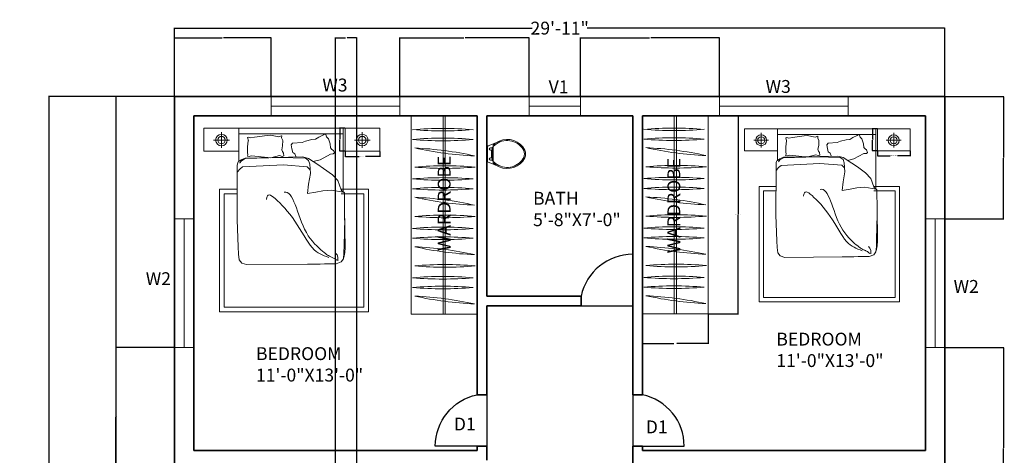
# Model space of a CAD drawing. Units: inches. Extents: x -53 to 406, y -526 to 46.
# Tile 2 of 2: x -53 to 406, y -157 to 46. Entities that reach past the tile are written whole.
import ezdxf

# ---------------------------------------------------------------- set-up
doc = ezdxf.new("R2010")
doc.units = ezdxf.units.IN
doc.header["$MEASUREMENT"] = 0
for name, color, linetype, lineweight in [('A-ANNO-DIMS', 2, 'Continuous', 18), ('A-ANNO-TEXT', 7, 'Continuous', 18), ('A-AREA-IDEN', 7, 'Continuous', 25), ('A-DOOR', 40, 'Continuous', 25), ('A-FLOR-CASE', 9, 'Continuous', 18), ('A-FURN', 8, 'Continuous', 13), ('A-GLAZ', 175, 'Continuous', 18), ('A-WALL', 7, 'Continuous', 35), ('WC-Detail_dwgmodels.com', 251, 'Continuous', 13), ('WC-Outline_dwgmodels.com', 250, 'Continuous', 18)]:
    doc.layers.add(name, color=color, linetype=linetype, lineweight=lineweight)
doc.styles.get("Standard").update_dxf_attribs({"font": 'arial.ttf'})
doc.dimstyles.get("Standard").update_dxf_attribs({"dimtxt": 0.18, "dimasz": 0.18, "dimexe": 0.18, "dimexo": 0.0625, "dimgap": 0.09, "dimtad": 0, "dimtih": 1, "dimtoh": 1, "dimdec": 0, "dimzin": 0, "dimdsep": 46, "dimlunit": 3, "dimtxsty": 'Standard', "dimcen": 0.09, "dimadec": 0, "dimazin": 0, "dimtfac": 1, "dimtdec": 0, "dimtofl": 0, "dimtmove": 0, "dimatfit": 3, "dimfxl": 1, "dimtolj": 1, "dimtzin": 0, "dimarcsym": 0})

# ---------------------------------------------------------------- blocks, each defined once
blk = doc.blocks.new('*D1')
at = {"layer": 'A-ANNO-DIMS', "color": 0, "lineweight": -2, "transparency": 16777216}
for p, q in [((19.43, 9.97), (19.43, 42.02)), ((19.61, 41.84), (186.15, 41.84)), ((378.25, 41.84), (211.71, 41.84)), ((378.43, 9.97), (378.43, 42.02))]:
    blk.add_line(p, q, dxfattribs=at)
at = {"layer": 'A-ANNO-DIMS', "color": 0, "transparency": 16777216}
for points in [[(19.61, 41.87), (19.61, 41.81), (19.43, 41.84)], [(378.25, 41.87), (378.25, 41.81), (378.43, 41.84)]]:
    blk.add_solid(points, dxfattribs=at)
at = {"layer": 'Defpoints', "color": 0, "transparency": 16777216}
for p in [(378.43, 41.84), (19.43, 9.91), (378.43, 9.91)]:
    blk.add_point(p, dxfattribs=at)
at = {"layer": 'A-ANNO-DIMS', "color": 0, "transparency": 16777216, "insert": (198.93, 41.84), "char_height": 6, "attachment_point": 5}
blk.add_mtext('\\A1;29\'-11"', dxfattribs=at)
blk = doc.blocks.new('*D2')
at = {"layer": 'A-ANNO-DIMS', "color": 0, "lineweight": -2, "transparency": 16777216}
for p, q in [((19.37, 9.91), (-39.35, 9.91)), ((-39.17, 9.73), (-39.17, -226.19)), ((-39.17, -468.41), (-39.17, -232.5)), ((19.37, -468.59), (-39.35, -468.59))]:
    blk.add_line(p, q, dxfattribs=at)
at = {"layer": 'A-ANNO-DIMS', "color": 0, "transparency": 16777216}
for points in [[(-39.2, 9.73), (-39.14, 9.73), (-39.17, 9.91)], [(-39.2, -468.41), (-39.14, -468.41), (-39.17, -468.59)]]:
    blk.add_solid(points, dxfattribs=at)
at = {"layer": 'Defpoints', "color": 0, "transparency": 16777216}
for p in [(19.43, 9.91), (-39.17, -468.59), (19.43, -468.59)]:
    blk.add_point(p, dxfattribs=at)
at = {"layer": 'A-ANNO-DIMS', "color": 0, "transparency": 16777216, "insert": (-39.17, -229.34), "char_height": 6, "attachment_point": 5}
blk.add_mtext('\\A1;39\'-11"', dxfattribs=at)
blk = doc.blocks.new('WIN-60IN-9IN-WALL')
for p, q in [((60, 9), (0, 9)), ((0, 9), (0, 0)), ((60, 0), (60, 9)), ((0, 4.5), (60, 4.5)), ((0, 0), (60, 0))]:
    blk.add_line(p, q)
blk = doc.blocks.new('VENT-24IN-9IN-WALL')
for p, q in [((24, 9), (0, 9)), ((0, 9), (0, 0)), ((24, 0), (24, 9)), ((0, 4.5), (24, 4.5)), ((0, 0), (24, 0))]:
    blk.add_line(p, q)
blk = doc.blocks.new('DOOR-24IN-SINGLE')
for p, q in [((24, 0), (24, 24)), ((0, 0), (24, 0))]:
    blk.add_line(p, q)
blk.add_arc((24, -0.52), 24.52, 90, 168.1877)
blk = doc.blocks.new('WARDROBE-HANGING')
for p, q in [((0, 0), (0, 92.26)), ((30.75, 92.26), (0, 92.26)), ((14.86, 0), (14.86, 92.26)), ((15.89, 0), (15.89, 92.26)), ((30.75, 0), (30.75, 92.26)), ((30.75, 0), (0, 0))]:
    blk.add_line(p, q)
for centre, start, end in [((14.76, -75.2), 85.0028, 94.9972), ((14.76, 247.2), 265.0028, 274.9972), ((14.76, -79.75), 85.0028, 94.9972), ((14.76, 242.64), 265.0028, 274.9972), ((36.65, 235.44), 257.508, 267.5023), ((-5.4, -84.2), 77.508, 87.5023), ((15.75, -92.64), 85.0028, 94.9972), ((15.75, 229.75), 265.0028, 274.9972), ((14.76, -98.18), 85.0028, 94.9972), ((14.76, 224.21), 265.0028, 274.9972), ((14.76, -102.74), 85.0028, 94.9972), ((14.76, 219.65), 265.0028, 274.9972), ((36.65, 212.45), 257.508, 267.5023), ((-5.4, -107.18), 77.508, 87.5023), ((15.75, -115.63), 85.0028, 94.9972), ((15.75, 206.76), 265.0028, 274.9972), ((14.76, -121.25), 85.0028, 94.9972), ((14.76, 201.14), 265.0028, 274.9972), ((14.76, -125.81), 85.0028, 94.9972), ((14.76, 196.58), 265.0028, 274.9972), ((-5.4, -130.25), 77.508, 87.5023), ((36.65, 189.38), 257.508, 267.5023), ((15.75, -138.7), 85.0028, 94.9972), ((15.75, 183.69), 265.0028, 274.9972), ((14.76, -144.24), 85.0028, 94.9972), ((14.76, 178.15), 265.0028, 274.9972), ((14.76, -148.79), 85.0028, 94.9972), ((14.76, 173.6), 265.0028, 274.9972), ((-5.4, -153.24), 77.508, 87.5023), ((36.65, 166.4), 257.508, 267.5023)]:
    blk.add_arc(centre, 161.81, start, end)
blk = doc.blocks.new('NIGHTSTAND-15IN')
for p, q in [((4.25, 4.91), (11.18, 4.91)), ((7.71, 8.38), (7.71, 1.45))]:
    blk.add_line(p, q)
blk.add_lwpolyline([(0, 0), (15.27, 0), (15.27, 10.18), (0, 10.18)], close=True)
for radius in [2.55, 1.63]:
    blk.add_circle((7.71, 4.91), radius)
blk = doc.blocks.new('NIGHTSTAND-16IN')
for p, q in [((4.52, 5.22), (11.88, 5.22)), ((8.2, 8.9), (8.2, 1.54))]:
    blk.add_line(p, q)
blk.add_lwpolyline([(0, 0), (16.23, 0), (16.23, 10.82), (0, 10.82)], close=True)
for radius in [2.71, 1.73]:
    blk.add_circle((8.2, 5.22), radius)
blk = doc.blocks.new('*D15')
at = {"layer": 'A-ANNO-DIMS', "color": 0, "lineweight": -2, "transparency": 16777216}
for p, q in [((268.25, 0.91), (282.2, 0.91)), ((282.02, 0.73), (282.02, -45.04)), ((282.02, -91.17), (282.02, -45.4)), ((268.25, -91.35), (282.2, -91.35))]:
    blk.add_line(p, q, dxfattribs=at)
at = {"layer": 'A-ANNO-DIMS', "color": 0, "transparency": 16777216}
for points in [[(281.99, 0.73), (282.05, 0.73), (282.02, 0.91)], [(281.99, -91.17), (282.05, -91.17), (282.02, -91.35)]]:
    blk.add_solid(points, dxfattribs=at)
at = {"layer": 'Defpoints', "color": 0, "transparency": 16777216}
for p in [(268.18, 0.91), (282.02, 0.91), (268.18, -91.35)]:
    blk.add_point(p, dxfattribs=at)
at = {"layer": 'A-ANNO-DIMS', "color": 0, "transparency": 16777216, "insert": (282.02, -45.22), "char_height": 0.18, "attachment_point": 5}
blk.add_mtext('\\A1;WARDROBE 7\'-8 1/2" TYP.', dxfattribs=at)
blk = doc.blocks.new('*D16')
at = {"layer": 'A-ANNO-DIMS', "color": 0, "lineweight": -2, "transparency": 16777216}
for p, q in [((237.43, -91.41), (237.43, -105.37)), ((268.18, -91.41), (268.18, -105.37)), ((237.61, -105.19), (252.17, -105.19)), ((268, -105.19), (253.45, -105.19))]:
    blk.add_line(p, q, dxfattribs=at)
at = {"layer": 'A-ANNO-DIMS', "color": 0, "transparency": 16777216}
for points in [[(237.61, -105.16), (237.61, -105.22), (237.43, -105.19)], [(268, -105.16), (268, -105.22), (268.18, -105.19)]]:
    blk.add_solid(points, dxfattribs=at)
at = {"layer": 'Defpoints', "color": 0, "transparency": 16777216}
for p in [(237.43, -91.35), (268.18, -91.35), (268.18, -105.19)]:
    blk.add_point(p, dxfattribs=at)
at = {"layer": 'A-ANNO-DIMS', "color": 0, "transparency": 16777216, "insert": (252.81, -105.19), "char_height": 0.18, "attachment_point": 5}
blk.add_mtext('\\A1;2\'-7" TYP.', dxfattribs=at)
blk = doc.blocks.new('*D17')
at = {"layer": 'A-ANNO-DIMS', "color": 0, "lineweight": -2, "transparency": 16777216}
for p, q in [((347.01, -15.4), (347.01, -17.81)), ((347.19, -17.63), (352.94, -17.63)), ((362.09, -17.63), (356.34, -17.63)), ((362.27, -15.4), (362.27, -17.81))]:
    blk.add_line(p, q, dxfattribs=at)
at = {"layer": 'A-ANNO-DIMS', "color": 0, "transparency": 16777216}
for points in [[(347.19, -17.6), (347.19, -17.66), (347.01, -17.63)], [(362.09, -17.6), (362.09, -17.66), (362.27, -17.63)]]:
    blk.add_solid(points, dxfattribs=at)
at = {"layer": 'Defpoints', "color": 0, "transparency": 16777216}
for p in [(347.01, -15.34), (347.01, -17.63), (362.27, -15.34)]:
    blk.add_point(p, dxfattribs=at)
at = {"layer": 'A-ANNO-DIMS', "color": 0, "transparency": 16777216, "insert": (354.64, -17.63), "char_height": 0.18, "attachment_point": 5}
blk.add_mtext('\\A1;NIGHTSTAND 1\'-3 1/2" TYP.', dxfattribs=at)
blk = doc.blocks.new('*D18')
at = {"layer": 'A-ANNO-DIMS', "color": 0, "lineweight": -2, "transparency": 16777216}
for p, q in [((346.95, -5.16), (344.54, -5.16)), ((344.72, -5.34), (344.72, -10.07)), ((344.72, -15.16), (344.72, -10.43)), ((346.95, -15.34), (344.54, -15.34))]:
    blk.add_line(p, q, dxfattribs=at)
at = {"layer": 'A-ANNO-DIMS', "color": 0, "transparency": 16777216}
for points in [[(344.69, -5.34), (344.75, -5.34), (344.72, -5.16)], [(344.69, -15.16), (344.75, -15.16), (344.72, -15.34)]]:
    blk.add_solid(points, dxfattribs=at)
at = {"layer": 'Defpoints', "color": 0, "transparency": 16777216}
for p in [(344.72, -5.16), (347.01, -5.16), (347.01, -15.34)]:
    blk.add_point(p, dxfattribs=at)
at = {"layer": 'A-ANNO-DIMS', "color": 0, "transparency": 16777216, "insert": (344.72, -10.25), "char_height": 0.18, "attachment_point": 5}
blk.add_mtext('\\A1;0\'-10" TYP.', dxfattribs=at)
blk = doc.blocks.new('*D19')
at = {"layer": 'A-ANNO-DIMS', "color": 0, "lineweight": -2, "transparency": 16777216}
for p, q in [((98.87, -15.63), (98.87, -18.18)), ((99.05, -18), (105.5, -18)), ((114.92, -18), (108.47, -18)), ((115.1, -15.63), (115.1, -18.18))]:
    blk.add_line(p, q, dxfattribs=at)
at = {"layer": 'A-ANNO-DIMS', "color": 0, "transparency": 16777216}
for points in [[(99.05, -17.97), (99.05, -18.03), (98.87, -18)], [(114.92, -17.97), (114.92, -18.03), (115.1, -18)]]:
    blk.add_solid(points, dxfattribs=at)
at = {"layer": 'Defpoints', "color": 0, "transparency": 16777216}
for p in [(98.87, -15.57), (98.87, -18), (115.1, -15.57)]:
    blk.add_point(p, dxfattribs=at)
at = {"layer": 'A-ANNO-DIMS', "color": 0, "transparency": 16777216, "insert": (106.98, -18), "char_height": 0.18, "attachment_point": 5}
blk.add_mtext('\\A1;NIGHTSTAND 1\'-4" TYP.', dxfattribs=at)
blk = doc.blocks.new('*D20')
at = {"layer": 'A-ANNO-DIMS', "color": 0, "lineweight": -2, "transparency": 16777216}
for p, q in [((98.81, -4.75), (96.26, -4.75)), ((96.44, -4.93), (96.44, -9.98)), ((96.44, -15.39), (96.44, -10.34)), ((98.81, -15.57), (96.26, -15.57))]:
    blk.add_line(p, q, dxfattribs=at)
at = {"layer": 'A-ANNO-DIMS', "color": 0, "transparency": 16777216}
for points in [[(96.41, -4.93), (96.47, -4.93), (96.44, -4.75)], [(96.41, -15.39), (96.47, -15.39), (96.44, -15.57)]]:
    blk.add_solid(points, dxfattribs=at)
at = {"layer": 'Defpoints', "color": 0, "transparency": 16777216}
for p in [(96.44, -4.75), (98.87, -4.75), (98.87, -15.57)]:
    blk.add_point(p, dxfattribs=at)
at = {"layer": 'A-ANNO-DIMS', "color": 0, "transparency": 16777216, "insert": (96.44, -10.16), "char_height": 0.18, "attachment_point": 5}
blk.add_mtext('\\A1;0\'-11" TYP.', dxfattribs=at)
blk = doc.blocks.new('*D22')
at = {"layer": 'A-ANNO-DIMS', "color": 0, "lineweight": -2, "transparency": 16777216}
for p, q in [((19.43, 9.97), (19.43, 37.44)), ((19.61, 37.26), (41.6, 37.26)), ((64.25, 37.26), (42.26, 37.26)), ((64.43, 9.97), (64.43, 37.44))]:
    blk.add_line(p, q, dxfattribs=at)
at = {"layer": 'A-ANNO-DIMS', "color": 0, "transparency": 16777216}
for points in [[(19.61, 37.29), (19.61, 37.23), (19.43, 37.26)], [(64.25, 37.29), (64.25, 37.23), (64.43, 37.26)]]:
    blk.add_solid(points, dxfattribs=at)
at = {"layer": 'Defpoints', "color": 0, "transparency": 16777216}
for p in [(64.43, 37.26), (19.43, 9.91), (64.43, 9.91)]:
    blk.add_point(p, dxfattribs=at)
at = {"layer": 'A-ANNO-DIMS', "color": 0, "transparency": 16777216, "insert": (41.93, 37.26), "char_height": 0.18, "attachment_point": 5}
blk.add_mtext('\\A1;3\'-9"', dxfattribs=at)
blk = doc.blocks.new('*D23')
at = {"layer": 'A-ANNO-DIMS', "color": 0, "lineweight": -2, "transparency": 16777216}
for p, q in [((124.43, 9.97), (124.43, 37.44)), ((124.61, 37.26), (154.23, 37.26)), ((184.5, 37.26), (154.88, 37.26)), ((184.68, 9.97), (184.68, 37.44))]:
    blk.add_line(p, q, dxfattribs=at)
at = {"layer": 'A-ANNO-DIMS', "color": 0, "transparency": 16777216}
for points in [[(124.61, 37.29), (124.61, 37.23), (124.43, 37.26)], [(184.5, 37.29), (184.5, 37.23), (184.68, 37.26)]]:
    blk.add_solid(points, dxfattribs=at)
at = {"layer": 'Defpoints', "color": 0, "transparency": 16777216}
for p in [(184.68, 37.26), (124.43, 9.91), (184.68, 9.91)]:
    blk.add_point(p, dxfattribs=at)
at = {"layer": 'A-ANNO-DIMS', "color": 0, "transparency": 16777216, "insert": (154.56, 37.26), "char_height": 0.18, "attachment_point": 5}
blk.add_mtext('\\A1;5\'-0"', dxfattribs=at)
blk = doc.blocks.new('*D24')
at = {"layer": 'A-ANNO-DIMS', "color": 0, "lineweight": -2, "transparency": 16777216}
for p, q in [((208.68, 9.97), (208.68, 37.44)), ((208.86, 37.26), (240.73, 37.26)), ((273.25, 37.26), (241.38, 37.26)), ((273.43, 9.97), (273.43, 37.44))]:
    blk.add_line(p, q, dxfattribs=at)
at = {"layer": 'A-ANNO-DIMS', "color": 0, "transparency": 16777216}
for points in [[(208.86, 37.29), (208.86, 37.23), (208.68, 37.26)], [(273.25, 37.29), (273.25, 37.23), (273.43, 37.26)]]:
    blk.add_solid(points, dxfattribs=at)
at = {"layer": 'Defpoints', "color": 0, "transparency": 16777216}
for p in [(273.43, 37.26), (208.68, 9.91), (273.43, 9.91)]:
    blk.add_point(p, dxfattribs=at)
at = {"layer": 'A-ANNO-DIMS', "color": 0, "transparency": 16777216, "insert": (241.06, 37.26), "char_height": 0.18, "attachment_point": 5}
blk.add_mtext('\\A1;5\'-5"', dxfattribs=at)
blk = doc.blocks.new('*D25')
at = {"layer": 'A-ANNO-DIMS', "color": 0, "lineweight": -2, "transparency": 16777216}
for p, q in [((378.49, 9.91), (405.96, 9.91)), ((405.78, 9.73), (405.78, -18.41)), ((405.78, -46.91), (405.78, -18.77)), ((378.49, -47.09), (405.96, -47.09))]:
    blk.add_line(p, q, dxfattribs=at)
at = {"layer": 'A-ANNO-DIMS', "color": 0, "transparency": 16777216}
for points in [[(405.75, 9.73), (405.81, 9.73), (405.78, 9.91)], [(405.75, -46.91), (405.81, -46.91), (405.78, -47.09)]]:
    blk.add_solid(points, dxfattribs=at)
at = {"layer": 'Defpoints', "color": 0, "transparency": 16777216}
for p in [(378.43, 9.91), (378.43, -47.09), (405.78, -47.09)]:
    blk.add_point(p, dxfattribs=at)
at = {"layer": 'A-ANNO-DIMS', "color": 0, "transparency": 16777216, "insert": (405.78, -18.59), "char_height": 0.18, "attachment_point": 5}
blk.add_mtext('\\A1;4\'-9"', dxfattribs=at)
blk = doc.blocks.new('*D26')
at = {"layer": 'A-ANNO-DIMS', "color": 0, "lineweight": -2, "transparency": 16777216}
for p, q in [((378.49, -107.09), (405.96, -107.09)), ((405.78, -107.27), (405.78, -153.82)), ((405.78, -200.73), (405.78, -154.18)), ((378.49, -200.91), (405.96, -200.91))]:
    blk.add_line(p, q, dxfattribs=at)
at = {"layer": 'A-ANNO-DIMS', "color": 0, "transparency": 16777216}
for points in [[(405.75, -107.27), (405.81, -107.27), (405.78, -107.09)], [(405.75, -200.73), (405.81, -200.73), (405.78, -200.91)]]:
    blk.add_solid(points, dxfattribs=at)
at = {"layer": 'Defpoints', "color": 0, "transparency": 16777216}
for p in [(378.43, -107.09), (378.43, -200.91), (405.78, -200.91)]:
    blk.add_point(p, dxfattribs=at)
at = {"layer": 'A-ANNO-DIMS', "color": 0, "transparency": 16777216, "insert": (405.78, -154), "char_height": 0.18, "attachment_point": 5}
blk.add_mtext('\\A1;7\'-10"', dxfattribs=at)
blk = doc.blocks.new('*D27')
at = {"layer": 'A-ANNO-DIMS', "color": 0, "lineweight": -2, "transparency": 16777216}
for p, q in [((19.37, -107.09), (-8.1, -107.09)), ((-7.92, -107.27), (-7.92, -139.26)), ((-7.92, -171.61), (-7.92, -139.63)), ((19.37, -171.79), (-8.1, -171.79))]:
    blk.add_line(p, q, dxfattribs=at)
at = {"layer": 'A-ANNO-DIMS', "color": 0, "transparency": 16777216}
for points in [[(-7.95, -107.27), (-7.89, -107.27), (-7.92, -107.09)], [(-7.95, -171.61), (-7.89, -171.61), (-7.92, -171.79)]]:
    blk.add_solid(points, dxfattribs=at)
at = {"layer": 'Defpoints', "color": 0, "transparency": 16777216}
for p in [(19.43, -107.09), (-7.92, -171.79), (19.43, -171.79)]:
    blk.add_point(p, dxfattribs=at)
at = {"layer": 'A-ANNO-DIMS', "color": 0, "transparency": 16777216, "insert": (-7.92, -139.44), "char_height": 0.18, "attachment_point": 5}
blk.add_mtext('\\A1;5\'-4 1/2"', dxfattribs=at)
blk = doc.blocks.new('*D33')
at = {"layer": 'A-ANNO-DIMS', "color": 0, "lineweight": -2, "transparency": 16777216}
for p, q in [((19.37, 9.91), (-8.1, 9.91)), ((-7.92, 9.73), (-7.92, -244.16)), ((-7.92, -498.41), (-7.92, -244.52)), ((164.87, -498.59), (-8.1, -498.59))]:
    blk.add_line(p, q, dxfattribs=at)
at = {"layer": 'A-ANNO-DIMS', "color": 0, "transparency": 16777216}
for points in [[(-7.95, 9.73), (-7.89, 9.73), (-7.92, 9.91)], [(-7.95, -498.41), (-7.89, -498.41), (-7.92, -498.59)]]:
    blk.add_solid(points, dxfattribs=at)
at = {"layer": 'Defpoints', "color": 0, "transparency": 16777216}
for p in [(19.43, 9.91), (-7.92, -498.59), (164.93, -498.59)]:
    blk.add_point(p, dxfattribs=at)
at = {"layer": 'A-ANNO-DIMS', "color": 0, "transparency": 16777216, "insert": (-7.92, -244.34), "char_height": 0.18, "attachment_point": 5}
blk.add_mtext('\\A1;42\'-4 1/2"', dxfattribs=at)
blk = doc.blocks.new('*D38')
at = {"layer": 'A-ANNO-DIMS', "color": 0, "lineweight": -2, "transparency": 16777216}
for p, q in [((94.43, -212.03), (94.43, 37.44)), ((94.61, 37.26), (99.03, 37.26)), ((104.25, 37.26), (99.83, 37.26)), ((104.43, -212.03), (104.43, 37.44))]:
    blk.add_line(p, q, dxfattribs=at)
at = {"layer": 'A-ANNO-DIMS', "color": 0, "transparency": 16777216}
for points in [[(94.61, 37.29), (94.61, 37.23), (94.43, 37.26)], [(104.25, 37.29), (104.25, 37.23), (104.43, 37.26)]]:
    blk.add_solid(points, dxfattribs=at)
at = {"layer": 'Defpoints', "color": 0, "transparency": 16777216}
for p in [(104.43, 37.26), (94.43, -212.09), (104.43, -212.09)]:
    blk.add_point(p, dxfattribs=at)
at = {"layer": 'A-ANNO-DIMS', "color": 0, "transparency": 16777216, "insert": (99.43, 37.26), "char_height": 0.18, "attachment_point": 5}
blk.add_mtext('\\A1;0\'-10"', dxfattribs=at)

msp = doc.modelspace()

# ---------------------------------------------------------------- linework, layer by layer
at = {"layer": 'A-FURN'}
for p, q in [((49.37, -20.4), (49.37, -4.75)), ((53.85, -10.71), (53.43, -9.13)), ((64.08, -8.03), (62.61, -8.19)), ((68.07, -8.86), (64.08, -8.03)), ((69.3, -8.41), (68.07, -8.86)), ((69.41, -8.44), (69.3, -8.41)), ((69.41, -8.44), (69.32, -9.35)), ((69.41, -8.44), (69.32, -9.35)), ((85.13, -9.96), (86.65, -8.94)), ((85.13, -9.96), (86.65, -8.94)), ((86.65, -8.94), (88.8, -7.94)), ((90.26, -8.79), (91.12, -9.73)), ((300.43, -19.89), (300.43, -5.16)), ((314.27, -8.24), (312.89, -8.4)), ((318.03, -9.02), (314.27, -8.24)), ((319.18, -8.6), (318.03, -9.02)), ((319.29, -8.63), (319.18, -8.6)), ((319.29, -8.63), (319.21, -9.48)), ((319.29, -8.63), (319.21, -9.48)), ((334.08, -10.06), (335.51, -9.11)), ((334.08, -10.06), (335.51, -9.11)), ((335.51, -9.11), (337.53, -8.17)), ((338.9, -8.96), (339.71, -9.84)), ((69.32, -9.35), (69.81, -10.52)), ((69.79, -13.01), (69.35, -14.85)), ((69.81, -10.52), (69.79, -13.01)), ((74.37, -11.74), (78.94, -11.47)), ((78.94, -11.47), (80.49, -10.89)), ((80.49, -10.89), (83.42, -10.1)), ((83.42, -10.1), (85.13, -9.96)), ((91.12, -9.73), (91.94, -12.08)), ((91.94, -12.08), (92.14, -13.96)), ((304.64, -10.76), (304.25, -9.28)), ((319.21, -9.48), (319.67, -10.59)), ((319.65, -12.93), (319.23, -14.66)), ((319.67, -10.59), (319.65, -12.93)), ((323.96, -11.74), (328.26, -11.48)), ((328.26, -11.48), (329.71, -10.93)), ((329.71, -10.93), (332.47, -10.19)), ((332.47, -10.19), (334.08, -10.06)), ((339.71, -9.84), (340.48, -12.05)), ((340.48, -12.05), (340.68, -13.83)), ((68.26, -17.59), (64.32, -18.6)), ((69.51, -17.99), (68.26, -17.59)), ((69.35, -14.85), (69.66, -15.73)), ((70.28, -17.74), (69.51, -17.99)), ((69.66, -15.73), (70.2, -16.44)), ((70.2, -16.44), (70.28, -17.74)), ((92.05, -16.9), (87.25, -19.6)), ((93.36, -16.85), (92.05, -16.9)), ((92.14, -13.96), (92.73, -14.69)), ((92.73, -14.69), (93.48, -15.16)), ((93.99, -16.36), (93.36, -16.85)), ((93.48, -15.16), (93.99, -16.36)), ((318.21, -17.24), (314.5, -18.19)), ((319.38, -17.61), (318.21, -17.24)), ((319.23, -14.66), (319.52, -15.5)), ((320.1, -17.38), (319.38, -17.61)), ((319.52, -15.5), (320.03, -16.16)), ((320.03, -16.16), (320.1, -17.38)), ((340.59, -16.6), (336.07, -19.13)), ((341.82, -16.55), (340.59, -16.6)), ((340.68, -13.83), (341.23, -14.51)), ((341.23, -14.51), (341.94, -14.96)), ((342.42, -16.08), (341.82, -16.55)), ((341.94, -14.96), (342.42, -16.08)), ((48.68, -21.48), (48.61, -22.23)), ((48.61, -22.23), (48.64, -24)), ((299.79, -20.9), (299.72, -21.61)), ((299.72, -21.61), (299.74, -23.27)), ((48.64, -24), (48.54, -47.57)), ((299.74, -23.27), (299.65, -45.44)), ((97.98, -34.63), (98.08, -34.58)), ((98.7, -43.69), (98.63, -36.05)), ((346.17, -33.27), (346.26, -33.23)), ((346.85, -41.8), (346.78, -34.61)), ((98.88, -60.43), (98.7, -43.69)), ((299.65, -45.44), (300.13, -57.33)), ((346.9, -44.89), (346.59, -56.79)), ((347.01, -57.55), (346.85, -41.8)), ((48.54, -47.57), (49.04, -60.2)), ((98.76, -46.98), (98.43, -59.63)), ((98.43, -59.63), (98.36, -62.94)), ((300.13, -57.33), (300.29, -60.45)), ((346.59, -56.79), (346.53, -59.91)), ((346.88, -59.74), (347.01, -57.55)), ((49.04, -60.2), (49.22, -63.51)), ((49.22, -63.51), (49.52, -66.23)), ((95.15, -63.87), (94.36, -63.04)), ((95.51, -64.98), (95.15, -63.87)), ((98.36, -62.94), (98.14, -65.67)), ((98.28, -65.17), (98.74, -62.76)), ((98.74, -62.76), (98.88, -60.43)), ((300.29, -60.45), (300.57, -63.01)), ((300.57, -63.01), (301.69, -64.37)), ((343.5, -60.78), (342.76, -60)), ((345.24, -63.87), (343.09, -64.66)), ((343.84, -61.83), (343.5, -60.78)), ((343.91, -63.34), (343.84, -61.83)), ((346.32, -62.48), (345.24, -63.87)), ((346.53, -59.91), (346.32, -62.48)), ((346.45, -62.01), (346.88, -59.74)), ((49.52, -66.23), (50.71, -67.68)), ((50.71, -67.68), (53.02, -68.45)), ((81.43, -68.15), (53.02, -68.45)), ((81.43, -68.15), (87.24, -68.15)), ((87.24, -68.15), (89.29, -67.99)), ((89.29, -67.99), (94.71, -67.99)), ((97, -67.15), (94.71, -67.99)), ((95.58, -66.59), (95.51, -64.98)), ((98.14, -65.67), (97, -67.15)), ((301.69, -64.37), (303.86, -65.1)), ((330.6, -64.81), (303.86, -65.1)), ((330.6, -64.81), (336.06, -64.81)), ((336.06, -64.81), (337.99, -64.67)), ((337.99, -64.67), (343.09, -64.66))]:
    msp.add_line(p, q, dxfattribs=at)
for points in [[(49.37, -4.75), (98.06, -4.75), (98.06, -34.54)], [(98.06, -7.45), (49.37, -7.45)], [(62.61, -8.19), (56.72, -9.07), (55.01, -9.36), (53.99, -9.04), (53.43, -9.13)], [(90.26, -8.79), (89.95, -7.79), (89.3, -7.59), (88.8, -7.94)], [(300.43, -5.16), (346.25, -5.16), (346.25, -33.19)], [(346.25, -7.71), (300.43, -7.71)], [(312.89, -8.4), (307.34, -9.23), (305.74, -9.5), (304.78, -9.19), (304.25, -9.28)], [(338.9, -8.96), (338.61, -8.02), (338, -7.83), (337.53, -8.17)], [(62.84, -18.5), (56.91, -17.88), (55.19, -17.67), (54.19, -18.04), (53.36, -17.94), (53.59, -17.28), (53.46, -16.16), (53.42, -13.55), (53.79, -10.71)], [(74.37, -11.74), (73.74, -12.64), (74.04, -14.52), (74.49, -16.17), (75.4, -16.7), (75.92, -18.05), (75.93, -18.3)], [(313.1, -18.1), (307.53, -17.52), (305.91, -17.32), (304.97, -17.67), (304.19, -17.57), (304.4, -16.95), (304.28, -15.89), (304.24, -13.44), (304.59, -10.76)], [(323.96, -11.74), (323.36, -12.58), (323.65, -14.35), (324.07, -15.91), (324.92, -16.4), (325.42, -17.68), (325.42, -17.91)], [(49.78, -20.11), (50.45, -19.53), (52.27, -18.77), (79.17, -18.24), (81.87, -18.93), (86.19, -21.8), (88.91, -23.6), (92.99, -26.59), (95.59, -29.25), (97.13, -33.5), (97.88, -34.62)], [(346.25, -33.29), (341.11, -32.39), (337.32, -32.68), (334.23, -33.3), (330.55, -33.82), (331.05, -29.81), (331.87, -25.15), (331.51, -21.03), (330.98, -19.36), (329.63, -18.41), (318.77, -18.11), (303.16, -18.58), (301.57, -19.53), (300.89, -20.46), (300.81, -20.54)], [(300.82, -19.62), (301.45, -19.07), (303.16, -18.35), (328.47, -17.85), (331.01, -18.5), (335.08, -21.2), (337.63, -22.89), (341.47, -25.71), (343.92, -28.21), (345.37, -32.21), (346.08, -33.26)], [(48.7, -21.43), (48.86, -20.92), (49.09, -20.53), (49.37, -20.4), (49.68, -20.12), (49.73, -20.11)], [(82.46, -24.03), (81.24, -22.79), (70.26, -21.86), (67.06, -22.04), (51.16, -22.84), (49.82, -23.85), (48.8, -25.21)], [(98.07, -34.65), (92.61, -33.7), (88.58, -34), (85.29, -34.66), (81.38, -35.21), (81.91, -30.95), (82.79, -25.99), (82.4, -21.62), (81.83, -19.85), (80.4, -18.83), (68.86, -18.52), (52.27, -19.01), (50.58, -20.02), (49.86, -21.01), (49.77, -21.1)], [(87.25, -19.6), (84.06, -20.38)], [(299.81, -20.85), (299.95, -20.38), (300.17, -20.01), (300.43, -19.89), (300.73, -19.62), (300.77, -19.61)], [(331.57, -23.3), (330.42, -22.13), (320.09, -21.26), (317.07, -21.43), (302.11, -22.18), (300.85, -23.13), (299.9, -24.41)], [(336.07, -19.13), (333.07, -19.87)], [(345.26, -31.93), (357.24, -31.93), (357.24, -85.72), (291.92, -85.72), (291.92, -31.93), (299.71, -31.93)], [(97.02, -33.2), (109.75, -33.2), (109.75, -90.37), (40.32, -90.37), (40.32, -33.2), (48.6, -33.2)], [(97.02, -35.36), (107.59, -35.36), (107.59, -88.21), (42.49, -88.21), (42.49, -35.36), (48.6, -35.36)], [(91.26, -65.14), (90.22, -64.68), (89.22, -64.27), (88.24, -63.85), (87.28, -63.4), (86.34, -62.87), (85.41, -62.24), (84.48, -61.47), (83.55, -60.51), (82.63, -59.35), (81.69, -58.01), (80.73, -56.53), (79.76, -54.93), (78.75, -53.26), (77.72, -51.55), (76.64, -49.83), (75.53, -48.14), (74.36, -46.51), (73.17, -44.96), (71.97, -43.49), (70.77, -42.11), (69.6, -40.85), (68.48, -39.69), (67.42, -38.67), (66.45, -37.78), (65.58, -37.04), (64.8, -36.47), (64.13, -36.1), (63.56, -35.95), (63.08, -36.04), (62.7, -36.4), (62.41, -37.05), (62.22, -38.02)], [(95.1, -66.41), (94.65, -66.07), (94.24, -65.79), (93.87, -65.55), (93.52, -65.36), (93.19, -65.19), (92.88, -65.04), (92.57, -64.91), (92.25, -64.77), (91.92, -64.62), (91.57, -64.44), (91.19, -64.23), (90.76, -63.97), (90.27, -63.65), (89.71, -63.25), (89.08, -62.76), (88.35, -62.18), (87.53, -61.48), (86.63, -60.66), (85.68, -59.74), (84.69, -58.71), (83.69, -57.57), (82.7, -56.32), (81.75, -54.96), (80.86, -53.5), (80.05, -51.93), (79.3, -50.3), (78.61, -48.61), (77.97, -46.91), (77.37, -45.21), (76.79, -43.55), (76.22, -41.96), (75.65, -40.46), (75.08, -39.09), (74.49, -37.85), (73.89, -36.79), (73.26, -35.91), (72.62, -35.24), (71.94, -34.8), (71.24, -34.61), (70.5, -34.69)], [(98.63, -35.98), (98.55, -34.92), (98.24, -34.61), (98.06, -34.54)], [(345.26, -33.96), (355.21, -33.96), (355.21, -83.69), (293.96, -83.69), (293.96, -33.96), (299.71, -33.96)], [(339.84, -61.98), (338.87, -61.55), (337.93, -61.16), (337, -60.77), (336.1, -60.34), (335.22, -59.85), (334.34, -59.25), (333.47, -58.52), (332.6, -57.62), (331.72, -56.53), (330.84, -55.27), (329.94, -53.88), (329.02, -52.37), (328.08, -50.8), (327.1, -49.19), (326.09, -47.57), (325.04, -45.98), (323.95, -44.45), (322.83, -42.99), (321.7, -41.61), (320.57, -40.31), (319.47, -39.12), (318.41, -38.04), (317.42, -37.07), (316.5, -36.24), (315.68, -35.54), (314.95, -35.01), (314.32, -34.66), (313.78, -34.52), (313.33, -34.6), (312.98, -34.94), (312.7, -35.56), (312.52, -36.47)], [(343.46, -63.18), (343.03, -62.86), (342.65, -62.59), (342.3, -62.37), (341.97, -62.18), (341.66, -62.03), (341.37, -61.89), (341.08, -61.76), (340.78, -61.63), (340.47, -61.49), (340.14, -61.32), (339.78, -61.13), (339.37, -60.88), (338.91, -60.58), (338.39, -60.2), (337.79, -59.74), (337.11, -59.19), (336.34, -58.53), (335.49, -57.77), (334.59, -56.9), (333.66, -55.93), (332.72, -54.85), (331.8, -53.68), (330.9, -52.4), (330.06, -51.03), (329.3, -49.56), (328.59, -48.01), (327.95, -46.43), (327.34, -44.82), (326.78, -43.23), (326.23, -41.67), (325.7, -40.17), (325.16, -38.76), (324.62, -37.47), (324.07, -36.31), (323.5, -35.3), (322.91, -34.48), (322.3, -33.85), (321.67, -33.43), (321.01, -33.25), (320.31, -33.33)], [(346.78, -34.54), (346.7, -33.55), (346.42, -33.25), (346.25, -33.19)]]:
    msp.add_lwpolyline(points, dxfattribs=at)
at = {"layer": 'A-WALL'}
for p, q in [((19.43, 9.91), (19.43, -468.59)), ((19.43, 9.91), (378.43, 9.91)), ((378.43, 9.91), (378.43, -468.59)), ((28.43, 0.91), (160.43, 0.91)), ((28.43, 0.91), (28.43, -155.09)), ((160.43, 0.91), (160.43, -129.09)), ((164.93, 0.91), (164.93, -83.09)), ((164.93, 0.91), (232.93, 0.91)), ((232.93, 0.91), (232.93, -129.09)), ((237.43, 0.91), (237.43, -129.09)), ((237.43, 0.91), (369.43, 0.91)), ((369.43, 0.91), (369.43, -155.09)), ((164.93, -83.09), (208.93, -83.09)), ((208.93, -87.59), (208.93, -83.09)), ((164.93, -87.59), (208.93, -87.59)), ((164.93, -87.59), (164.93, -129.09)), ((161.67, -129.09), (160.43, -129.09)), ((161.67, -129.09), (164.93, -129.09)), ((235.18, -129.09), (232.93, -129.09)), ((235.18, -129.09), (237.43, -129.09)), ((28.43, -155.09), (160.43, -155.09)), ((160.43, -153.09), (164.93, -153.09)), ((160.43, -153.09), (160.43, -155.09)), ((164.93, -153.09), (164.93, -159.59)), ((237.43, -153.09), (232.93, -153.09)), ((232.93, -153.09), (232.93, -308.09)), ((237.43, -153.09), (237.43, -155.09)), ((237.43, -155.09), (369.43, -155.09))]:
    msp.add_line(p, q, dxfattribs=at)
at = {"layer": 'WC-Detail_dwgmodels.com'}
for p, q in [((167.96, -13.35), (167.96, -12.61)), ((167.96, -21.08), (167.96, -20.33))]:
    msp.add_line(p, q, dxfattribs=at)
for points in [[(167.42, -13.96, -0.022712), (167.96, -13.35, -0.162618)], [(167.96, -12.61, -0.040937), (169.17, -11.64, -0.163732)], [(167.42, -13.96), (166.68, -13.96, 1), (166.68, -15.09), (167.06, -15.09)], [(167.42, -16.84), (167.42, -13.96, -0.476108)], [(167.42, -16.84), (167.42, -19.72, 0.022712)], [(167.42, -19.72), (166.68, -19.72, -1), (166.68, -18.59), (167.06, -18.59)], [(167.42, -19.72, 0.022712), (167.96, -20.33, 0.162618)], [(167.96, -21.08, 0.040937), (169.17, -22.04, 0.163732)]]:
    msp.add_lwpolyline(points, format="xyb", dxfattribs=at)
for points in [[(167.06, -15.09), (167.06, -18.59)], [(167.06, -15.09), (167.42, -15.09)], [(167.06, -18.59), (167.42, -18.59)]]:
    msp.add_lwpolyline(points, dxfattribs=at)
at = {"layer": 'WC-Outline_dwgmodels.com'}
for p in [(167.96, -13.35), (167.96, -20.33)]:
    msp.add_line(p, (167.96, -16.84), dxfattribs=at)
for points in [[(165.27, -16.84), (165.27, -13.45, -0.31031), (165.55, -13.04), (169.17, -11.64, -0.209071)], [(167.96, -13.35, -0.448546), (181.33, -13.84, -0.162618), (182.49, -16.84, -0.470877)], [(169.17, -11.64, -0.383919), (181.74, -13.51, -0.163732), (183.02, -16.84, -0.359733)], [(165.27, -16.84), (165.27, -20.23, 0.31031), (165.55, -20.65), (169.17, -22.04, 0.209071)], [(168.32, -20.69, 0.431639), (181.33, -19.84, 0.162618), (182.49, -16.84, 0.470877)], [(169.17, -22.04, 0.383919), (181.74, -20.18, 0.163732), (183.02, -16.84, 0.359733)], [(167.96, -20.33, 0.014165), (168.32, -20.69, 0.162618)]]:
    msp.add_lwpolyline(points, format="xyb", dxfattribs=at)

# ---------------------------------------------------------------- block references
at = {"layer": 'A-DOOR'}
msp.add_blockref('DOOR-24IN-SINGLE', (208.93, -87.59), dxfattribs=at)
at = {"layer": 'A-DOOR', "extrusion": (0, 0, -1), "zscale": -1, "rotation": 270}
msp.add_blockref('DOOR-24IN-SINGLE', (-164.93, -129.09), dxfattribs=at)
at = {"layer": 'A-DOOR', "rotation": 270.0000000000001}
msp.add_blockref('DOOR-24IN-SINGLE', (232.93, -129.09), dxfattribs=at)
at = {"layer": 'A-FLOR-CASE'}
for p in [(129.68, -91.51), (237.43, -91.35)]:
    msp.add_blockref('WARDROBE-HANGING', p, dxfattribs=at)
at = {"layer": 'A-FURN'}
for name, p in [('NIGHTSTAND-16IN', (33.08, -15.57)), ('NIGHTSTAND-15IN', (285.11, -15.34))]:
    msp.add_blockref(name, p, dxfattribs=at)
at = {"layer": 'A-FURN', "extrusion": (0, 0, -1), "zscale": -1}
for name, p in [('NIGHTSTAND-16IN', (-115.1, -15.57)), ('NIGHTSTAND-15IN', (-362.27, -15.34))]:
    msp.add_blockref(name, p, dxfattribs=at)
at = {"layer": 'A-GLAZ'}
for name, p in [('WIN-60IN-9IN-WALL', (64.43, 0.91)), ('VENT-24IN-9IN-WALL', (184.68, 0.91)), ('WIN-60IN-9IN-WALL', (273.43, 0.91))]:
    msp.add_blockref(name, p, dxfattribs=at)
for p, rotation in [((28.43, -107.09), 90), ((378.43, -107.09), 89.99999999999969)]:
    msp.add_blockref('WIN-60IN-9IN-WALL', p, dxfattribs=dict(at, rotation=rotation))

# ---------------------------------------------------------------- texts
at = {"layer": 'A-ANNO-TEXT', "char_height": 6, "attachment_point": 1}
for s, insert in [('W3', (88.31, 18.3)), ('V1', (193.77, 17.45)), ('W3', (294.89, 17.64)), ('W2', (6.02, -71.99)), ('W2', (382.5, -75.6))]:
    msp.add_mtext(s, dxfattribs=dict(at, insert=insert))
at = {"layer": 'A-ANNO-TEXT', "char_height": 6, "attachment_point": 1, "rotation": 90}
for insert in [(142.07, -62.11), (249.12, -63.17)]:
    msp.add_mtext('WARDROBE', dxfattribs=dict(at, insert=insert))
at = {"layer": 'A-ANNO-TEXT', "char_height": 6, "attachment_point": 1}
for insert in [(149.6, -139.76), (239.05, -141.09)]:
    msp.add_mtext_dynamic_manual_height_columns('D1', width=0.3418, gutter_width=1, heights=[0], dxfattribs=dict(at, insert=insert))
at = {"layer": 'A-AREA-IDEN', "char_height": 6, "attachment_point": 1}
for s, insert in [('BATH\\P5\'-8"X7\'-0"', (186.51, -34.49)), ('BEDROOM\\P11\'-0"X13\'-0"', (299.89, -100.17)), ('BEDROOM\\P11\'-0"X13\'-0"', (57.38, -106.93))]:
    msp.add_mtext(s, dxfattribs=dict(at, insert=insert))

# ---------------------------------------------------------------- dimensions: what is measured, and where the dimension line sits
at = {"layer": 'A-ANNO-DIMS'}
for base, p1, p2, override, picture, middle in [((378.43, 41.84), (19.43, 9.91), (378.43, 9.91), {"dimtxt": 6, "dimclrd": 0, "dimclre": 0, "dimclrt": 0}, '*D1', (198.93, 41.84)), ((64.43, 37.26), (19.43, 9.91), (64.43, 9.91), {"dimdec": 1, "dimlfac": 1, "dimrnd": 0, "dimzin": 1, "dimdsep": 46, "dimlunit": 4, "dimfrac": 2}, '*D22', (41.93, 37.26)), ((104.43, 37.26), (94.43, -212.09), (104.43, -212.09), {"dimdec": 1, "dimlfac": 1, "dimrnd": 0, "dimzin": 1, "dimdsep": 46, "dimlunit": 4, "dimfrac": 2}, '*D38', (99.43, 37.26)), ((184.6798, 37.2588), (124.4311, 9.9088), (184.6798, 9.9088), {"dimdec": 1, "dimlfac": 1, "dimrnd": 0, "dimzin": 1, "dimdsep": 46, "dimlunit": 4, "dimfrac": 2}, '*D23', (154.5554, 37.2588)), ((273.4311, 37.2588), (208.6798, 9.9088), (273.4311, 9.9088), {"dimdec": 1, "dimlfac": 1, "dimrnd": 0, "dimzin": 1, "dimdsep": 46, "dimlunit": 4, "dimfrac": 2}, '*D24', (241.0554, 37.2588))]:
    dim = msp.add_linear_dim(base=base, p1=p1, p2=p2, dimstyle='Standard', override=override, dxfattribs=at)
    dim.commit()
    dim.dimension.update_dxf_attribs({"geometry": picture, "text_midpoint": middle})
for base, p1, p2, override, picture, middle in [((-39.16606535, -468.59119586), (19.43111134, 9.90880414), (19.43111134, -468.59119586), {"dimtxt": 6, "dimclrd": 0, "dimclre": 0, "dimclrt": 0}, '*D2', (-39.16606535, -229.34119586)), ((-7.92, -498.59), (19.43, 9.91), (164.93, -498.59), {"dimdec": 1, "dimlfac": 1, "dimrnd": 0, "dimzin": 1, "dimdsep": 46, "dimlunit": 4, "dimfrac": 2}, '*D33', (-7.92, -244.34)), ((405.78, -47.09), (378.43, 9.91), (378.43, -47.09), {"dimdec": 1, "dimlfac": 1, "dimrnd": 0, "dimzin": 1, "dimdsep": 46, "dimlunit": 4, "dimfrac": 2}, '*D25', (405.78, -18.59)), ((-7.92, -171.79), (19.43, -107.09), (19.43, -171.79), {"dimdec": 1, "dimlfac": 1, "dimrnd": 0, "dimzin": 1, "dimdsep": 46, "dimlunit": 4, "dimfrac": 2}, '*D27', (-7.92, -139.44)), ((405.78, -200.91), (378.43, -107.09), (378.43, -200.91), {"dimdec": 1, "dimlfac": 1, "dimrnd": 0, "dimzin": 1, "dimdsep": 46, "dimlunit": 4, "dimfrac": 2}, '*D26', (405.78, -154))]:
    dim = msp.add_linear_dim(base=base, p1=p1, p2=p2, angle=90, dimstyle='Standard', override=override, dxfattribs=at)
    dim.commit()
    dim.dimension.update_dxf_attribs({"geometry": picture, "text_midpoint": middle})
for base, p1, p2, angle, text, picture, middle in [((282.02, 0.91), (268.18, -91.35), (268.18, 0.91), 90, 'WARDROBE <> TYP.', '*D15', (282.02, -45.22)), ((96.44, -4.75), (98.87, -15.57), (98.87, -4.75), 90, '<> TYP.', '*D20', (96.44, -10.16)), ((344.72, -5.16), (347.01, -15.34), (347.01, -5.16), 90, '<> TYP.', '*D18', (344.72, -10.25)), ((98.87, -18), (115.1, -15.57), (98.87, -15.57), 180, 'NIGHTSTAND <> TYP.', '*D19', (106.98, -18)), ((347.01, -17.63), (362.27, -15.34), (347.01, -15.34), 180, 'NIGHTSTAND <> TYP.', '*D17', (354.64, -17.63))]:
    dim = msp.add_linear_dim(base=base, p1=p1, p2=p2, angle=angle, text=text, dimstyle='Standard', override={"dimdec": 1, "dimlfac": 1, "dimrnd": 0, "dimzin": 1, "dimdsep": 46, "dimlunit": 4, "dimfrac": 2}, dxfattribs=at)
    dim.commit()
    dim.dimension.update_dxf_attribs({"geometry": picture, "text_midpoint": middle})
dim = msp.add_linear_dim(base=(268.1835, -105.1868), p1=(237.4311, -91.3482), p2=(268.1835, -91.3482), text='<> TYP.', dimstyle='Standard', override={"dimdec": 1, "dimlfac": 1, "dimrnd": 0, "dimzin": 1, "dimdsep": 46, "dimlunit": 4, "dimfrac": 2}, dxfattribs=at)
dim.commit()
dim.dimension.update_dxf_attribs({"geometry": '*D16', "text_midpoint": (252.8073, -105.1868)})

doc.saveas('drawing.dxf')
